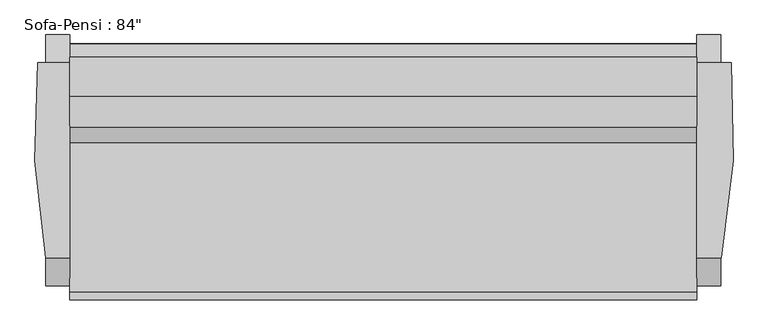
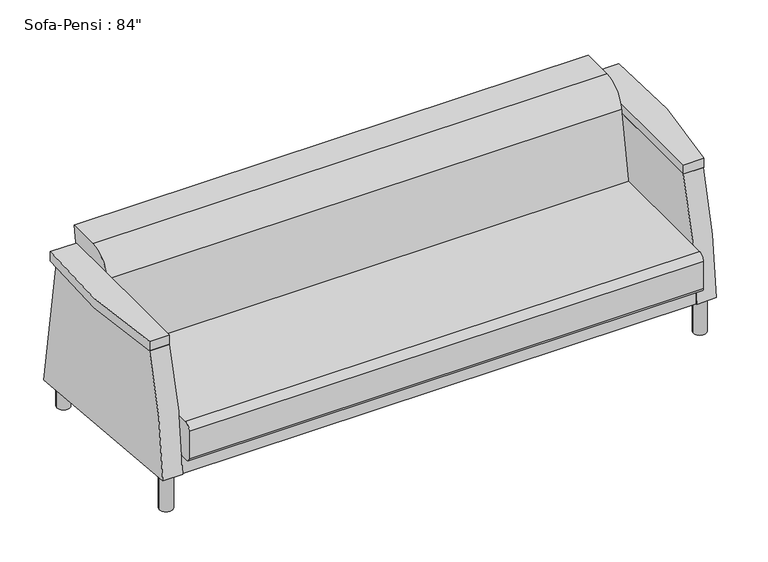
"""IFC4 building model written with IfcOpenShell, lengths in millimetres: furniture geometry."""

from ifc_helpers import new_model, si_unit, point, frame, frame_2d, origin, origin_with_axes, place, context, project, spatial, polyline, circle_curve, trimmed, segment, composite_curve, outline, extrude, source, transform, mapped, element, save


def furniture_aff9b2fb(model_context):
    return source(origin(), model_context, "Body", "SweptSolid", [
        extrude(outline(composite_curve([segment(trimmed(circle_curve(frame_2d((-750.09375, -53.0901639)), 25.4), [point((-775.49375, -53.0901639))], [point((-724.69375, -53.0901639))], False, "CARTESIAN"), True, "CONTINUOUS"), segment(trimmed(circle_curve(frame_2d((-750.09375, -53.0901639)), 25.4), [point((-724.69375, -53.0901639))], [point((-775.49375, -53.0901639))], False, "CARTESIAN"), True, "CONTINUOUS")], self_intersect=False)), origin_with_axes(), (0.0, 0.0, 1.0), 148.43125),
        extrude(outline(composite_curve([segment(trimmed(circle_curve(frame_2d((-750.09375, 632.7098361)), 25.4), [point((-775.49375, 632.7098361))], [point((-724.69375, 632.7098361))], False, "CARTESIAN"), True, "CONTINUOUS"), segment(trimmed(circle_curve(frame_2d((-750.09375, 632.7098361)), 25.4), [point((-724.69375, 632.7098361))], [point((-775.49375, 632.7098361))], False, "CARTESIAN"), True, "CONTINUOUS")], self_intersect=False)), origin_with_axes(), (0.0, 0.0, 1.0), 148.43125),
        extrude(outline(composite_curve([segment(trimmed(circle_curve(frame_2d((1307.30625, 632.7098361)), 25.4), [point((1281.90625, 632.7098361))], [point((1332.70625, 632.7098361))], False, "CARTESIAN"), True, "CONTINUOUS"), segment(trimmed(circle_curve(frame_2d((1307.30625, 632.7098361)), 25.4), [point((1332.70625, 632.7098361))], [point((1281.90625, 632.7098361))], False, "CARTESIAN"), True, "CONTINUOUS")], self_intersect=False)), origin_with_axes(), (0.0, 0.0, 1.0), 148.43125),
        extrude(outline(composite_curve([segment(trimmed(circle_curve(frame_2d((1307.30625, -53.0901639)), 25.4), [point((1281.90625, -53.0901639))], [point((1332.70625, -53.0901639))], False, "CARTESIAN"), True, "CONTINUOUS"), segment(trimmed(circle_curve(frame_2d((1307.30625, -53.0901639)), 25.4), [point((1332.70625, -53.0901639))], [point((1281.90625, -53.0901639))], False, "CARTESIAN"), True, "CONTINUOUS")], self_intersect=False)), origin_with_axes(), (0.0, 0.0, 1.0), 148.43125),
        extrude(outline(polyline([(1269.20625, 668.3047863), (1269.20625, -93.6952137), (-711.99375, -93.6952137), (-711.99375, 668.3047863), (1269.20625, 668.3047863)])), frame((0.0, 0.0, 148.0509954), z_axis=(0.0, 0.0, 1.0), x_axis=(1.0, 0.0, 0.0)), (0.0, 0.0, 1.0), 76.2),
        extrude(outline(composite_curve([segment(polyline([(-9.3943348, 626.0203985), (608.6917937, 626.0203985), (696.2098361, 79.844579), (-97.7900405, 149.3105671)]), True, "CONTINUOUS"), segment(trimmed(circle_curve(frame_2d((1499.9783711, 99.5888442)), 1598.5418814), [point((-97.7900405, 149.3105671))], [point((-9.3943348, 626.0203985))], False, "CARTESIAN"), True, "CONTINUOUS")], self_intersect=False)), frame((-788.19375, 0.0, 0.0), z_axis=(1.0, 0.0, 0.0), x_axis=(0.0, 1.0, 0.0)), (0.0, 0.0, 1.0), 76.2),
        extrude(outline(composite_curve([segment(polyline([(696.2098361, 79.844579), (-97.7900405, 149.3105671)]), True, "CONTINUOUS"), segment(trimmed(circle_curve(frame_2d((1499.9783711, 99.5888442)), 1598.5418814), [point((-97.7900405, 149.3105671))], [point((-9.3943348, 626.0203985))], False, "CARTESIAN"), True, "CONTINUOUS"), segment(polyline([(-9.3943348, 626.0203985), (608.6917937, 626.0203985), (696.2098361, 79.844579)]), True, "CONTINUOUS")], self_intersect=False)), frame((1269.20625, 0.0, 0.0), z_axis=(1.0, 0.0, 0.0), x_axis=(0.0, 1.0, 0.0)), (0.0, 0.0, 1.0), 76.2),
        extrude(outline(composite_curve([segment(trimmed(circle_curve(frame_2d((-116.5901639, 351.2509954)), 25.4), [point((-141.9901639, 351.2509954))], [point((-116.5901639, 376.6509954))], False, "CARTESIAN"), True, "CONTINUOUS"), segment(polyline([(-116.5901639, 376.6509954), (355.3895541, 376.6509954), (402.1988177, 642.1195211)]), True, "CONTINUOUS"), segment(trimmed(circle_curve(frame_2d((502.2552854, 624.4768662)), 101.6), [point((402.1988177, 642.1195211))], [point((502.2552854, 726.0768662))], False, "CARTESIAN"), True, "CONTINUOUS"), segment(polyline([(502.2552854, 726.0768662), (626.3344485, 726.0768662), (609.5377828, 620.1719187), (667.6541767, 224.2509954), (-126.1151639, 224.2509954)]), True, "CONTINUOUS"), segment(trimmed(circle_curve(frame_2d((-126.1151639, 240.1259954)), 15.875), [point((-126.1151639, 224.2509954))], [point((-141.9901639, 240.1259954))], False, "CARTESIAN"), True, "CONTINUOUS"), segment(polyline([(-141.9901639, 240.1259954), (-141.9901639, 351.2509954)]), True, "CONTINUOUS")], self_intersect=False)), frame((-711.99375, 0.0, 0.0), z_axis=(1.0, 0.0, 0.0), x_axis=(0.0, 1.0, 0.0)), (0.0, 0.0, 1.0), 1981.2),
        extrude(outline(composite_curve([segment(polyline([(-711.99375, -9.3943348), (-788.19375, -9.3943348)]), True, "CONTINUOUS"), segment(trimmed(circle_curve(frame_2d((1379.5527561, 389.2532985)), 2204.0972869), [point((-788.19375, -9.3943348))], [point((-813.59375, 608.6917935))], False, "CARTESIAN"), True, "CONTINUOUS"), segment(polyline([(-813.59375, 608.6917935), (-711.99375, 608.6917935), (-711.99375, -9.3943348)]), True, "CONTINUOUS")], self_intersect=False)), frame((0.0, 0.0, 626.0203985), z_axis=(0.0, 0.0, 1.0), x_axis=(1.0, 0.0, 0.0)), (0.0, 0.0, 1.0), 38.1),
        extrude(outline(composite_curve([segment(polyline([(1269.20625, -9.3943348), (1269.20625, 608.9395268), (1377.8864453, 608.9395268)]), True, "CONTINUOUS"), segment(trimmed(circle_curve(frame_2d((-821.3771494, 407.0073811)), 2208.514648), [point((1377.8864453, 608.9395268))], [point((1347.5273117, -9.3943348))], False, "CARTESIAN"), True, "CONTINUOUS"), segment(polyline([(1347.5273117, -9.3943348), (1269.20625, -9.3943348)]), True, "CONTINUOUS")], self_intersect=False)), frame((0.0, 0.0, 626.0203985), z_axis=(0.0, 0.0, 1.0), x_axis=(1.0, 0.0, 0.0)), (0.0, 0.0, 1.0), 38.1),
    ])


if __name__ == "__main__":
    model = new_model("IFC4")
    model_context = context("Model", 3, world=origin())
    ifc_project = project(units=[si_unit("LENGTHUNIT", "METRE", prefix="MILLI")], contexts=[model_context])
    site = spatial("IfcSite", under=ifc_project)
    building = spatial("IfcBuilding", under=site)
    placement = place(None, origin())
    furniture_shape = furniture_aff9b2fb(model_context)
    element("IfcFurniture", 1, ObjectType="Sofa-Pensi : 84\"", at=placement, inside=building, context=model_context, shape_type="MappedRepresentation", body=[
        mapped(furniture_shape, transform((0.0, 0.0, 0.0), x_axis=(1.0, 0.0, 0.0), y_axis=(0.0, 1.0, 0.0), z_axis=(0.0, 0.0, 1.0))),
    ])
    save(model, "model.ifc")

# Revit data of these elements
# Type "Sofa-Pensi : 84\""
#   Assembly Code = "E2020200"
#   Length = 7' - 0"
#   Frame Material = Cherry
#   Seat Material = Linen, Beige
#   Feet Material = Steel, Chrome Plated
#   Default Elevation = 0
# Element 1 (IfcFurniture, "Sofa-Pensi : 84\"")
#   Materials on its faces: "Cherry", "Linen, Beige", "Steel, Chrome Plated"
# Materials
#   "Cherry": class "Wood", colour RGB 226 177 128, transparency 0, Description = "Prunus Serotina", Cost = 0
#   "Linen, Beige": class "Textile", colour RGB 249 239 230, transparency 0, Description = "Linen, beige", Cost = 0
#   "Steel, Chrome Plated": class "Metal", colour RGB 17 17 17, transparency 0, Description = "Chromiuim plated steel", Cost = 0
